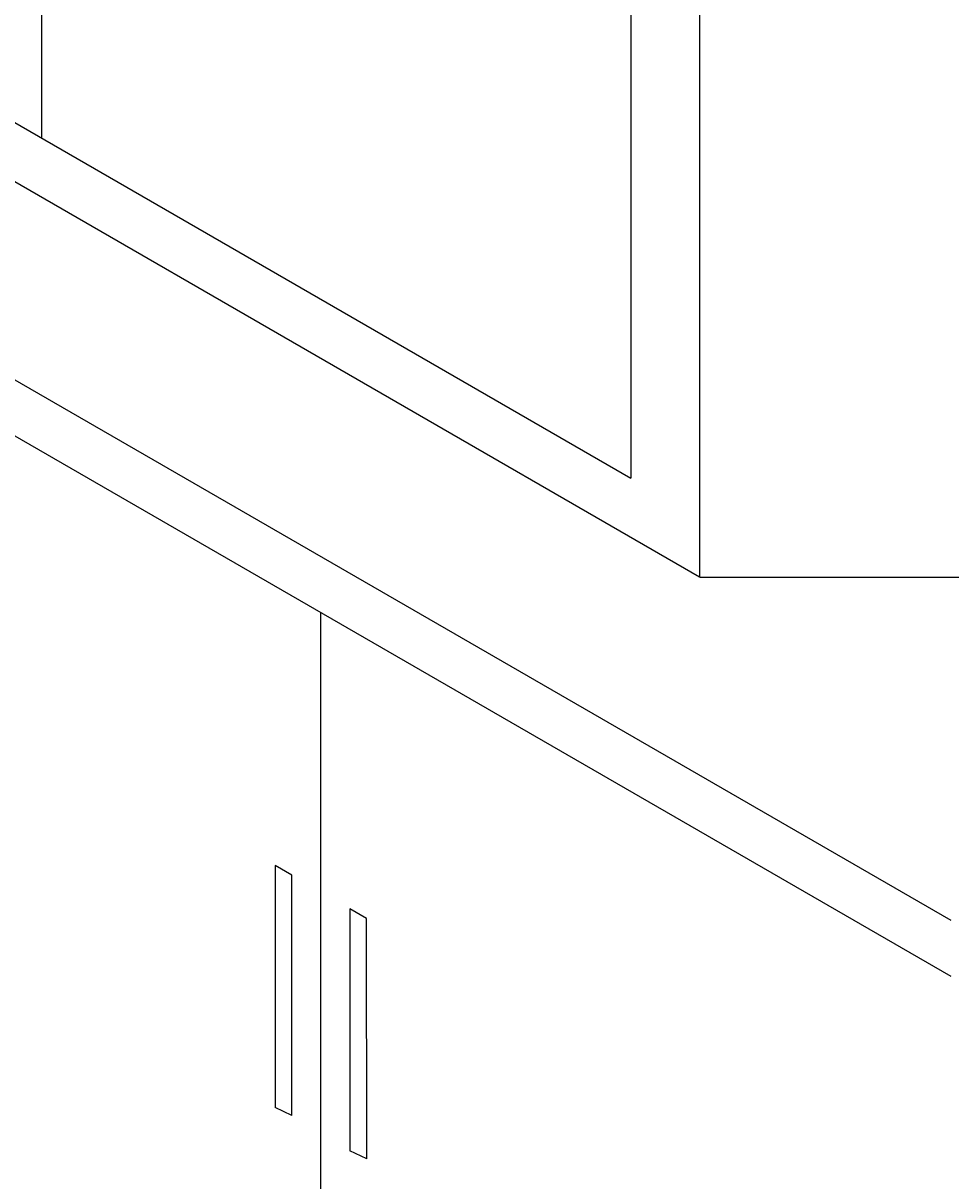
# Model space of a CAD drawing. Units: metres. Extents: x -2391 to 4922, y -635 to 4845.
# Tile 31 of 37: x 2198 to 3149, y 1238 to 2425. Entities that reach past the tile are written whole.
import ezdxf

# ---------------------------------------------------------------- set-up
doc = ezdxf.new("R2010")
doc.units = ezdxf.units.M
doc.header["$MEASUREMENT"] = 0
for name, color, linetype, lineweight in [('A-ANNO-DIMS', 2, 'Continuous', 18), ('A-FLOR-FIXT', 3, 'Continuous', 25), ('A-GLAZ', 4, 'Continuous', 25)]:
    doc.layers.add(name, color=color, linetype=linetype, lineweight=lineweight)
doc.styles.get("Standard").update_dxf_attribs({"font": 'arial.ttf'})
doc.dimstyles.get("Standard").update_dxf_attribs({"dimtxt": 5, "dimasz": 4, "dimexe": 0.18, "dimexo": 0.0625, "dimgap": 0.09, "dimtad": 0, "dimtih": 1, "dimtoh": 1, "dimdec": 0, "dimzin": 0, "dimdsep": 46, "dimtxsty": 'Standard', "dimcen": 0.09, "dimadec": 0, "dimazin": 0, "dimtfac": 1, "dimtdec": 0, "dimtofl": 0, "dimtmove": 0, "dimatfit": 3, "dimfxl": 1, "dimtolj": 1, "dimtzin": 0, "dimarcsym": 0})

# ---------------------------------------------------------------- blocks, each defined once
blk = doc.blocks.new('HANDLE-DOOR-256')
for p, q in [((0, 256.1), (0, 9.9)), ((0, 256.1), (17.1, 248)), ((17.1, 0), (17.1, 248)), ((0, 9.9), (17.1, 0))]:
    blk.add_line(p, q)
blk = doc.blocks.new('*D8')
at = {"layer": 'A-ANNO-DIMS', "color": 0, "lineweight": -2, "transparency": 16777216}
for p, q in [((-2047.3, 3005.2), (-2047.3, -631.4)), ((4577.8, 2350.2), (4577.8, -631.4)), ((-2043.3, -631.2), (1257.6, -631.2)), ((4573.8, -631.2), (1272.8, -631.2))]:
    blk.add_line(p, q, dxfattribs=at)
at = {"layer": 'A-ANNO-DIMS', "color": 0, "transparency": 16777216}
for points in [[(-2043.3, -630.6), (-2043.3, -631.9), (-2047.3, -631.2)], [(4573.8, -630.6), (4573.8, -631.9), (4577.8, -631.2)]]:
    blk.add_solid(points, dxfattribs=at)
at = {"layer": 'Defpoints', "color": 0, "transparency": 16777216}
for p in [(-2047.3, 3005.3), (4577.8, 2350.3), (4577.8, -631.2)]:
    blk.add_point(p, dxfattribs=at)
at = {"layer": 'A-ANNO-DIMS', "color": 0, "transparency": 16777216, "insert": (1265.2, -631.2), "char_height": 5, "attachment_point": 5}
blk.add_mtext('\\A1;6625', dxfattribs=at)
blk = doc.blocks.new('*D13')
at = {"layer": 'A-ANNO-DIMS', "color": 0, "lineweight": -2, "transparency": 16777216}
for p, q in [((2891.5, 2774), (3228.1, 2774)), ((3227.9, 2770), (3227.9, 2318)), ((3227.9, 1860.8), (3227.9, 2312.8)), ((2891.5, 1856.8), (3228.1, 1856.8))]:
    blk.add_line(p, q, dxfattribs=at)
at = {"layer": 'A-ANNO-DIMS', "color": 0, "transparency": 16777216}
for points in [[(3227.3, 2770), (3228.6, 2770), (3227.9, 2774)], [(3227.3, 1860.8), (3228.6, 1860.8), (3227.9, 1856.8)]]:
    blk.add_solid(points, dxfattribs=at)
at = {"layer": 'Defpoints', "color": 0, "transparency": 16777216}
for p in [(2891.4, 2774), (2891.4, 1856.8), (3227.9, 1856.8)]:
    blk.add_point(p, dxfattribs=at)
at = {"layer": 'A-ANNO-DIMS', "color": 0, "transparency": 16777216, "insert": (3227.9, 2315.4), "char_height": 5, "attachment_point": 5}
blk.add_mtext('\\A1;917.2', dxfattribs=at)

msp = doc.modelspace()

# ---------------------------------------------------------------- linework, layer by layer
at = {"layer": 'A-FLOR-FIXT'}
for p, q in [((550.7419, 3005.2763), (3148.8181, 1505.2763)), ((546.8938, 2950.1416), (3148.8181, 1447.9199)), ((2503.0469, 1820.756), (2503.0469, 998.1124))]:
    msp.add_line(p, q, dxfattribs=at)
at = {"layer": 'A-GLAZ'}
for p, q in [((2217.2021, 3091.6502), (2217.2021, 2306.7949)), ((2891.4324, 2773.9801), (2891.4324, 1856.8211)), ((2820.8768, 2743.1184), (2820.8768, 1958.2631)), ((1573.5273, 2678.4207), (2820.8768, 1958.2631)), ((2891.4324, 1856.8211), (1496.0309, 2662.4566))]:
    msp.add_line(p, q, dxfattribs=at)

# ---------------------------------------------------------------- block references
at = {"layer": 'A-FLOR-FIXT', "rotation": 180.0273381069543}
for p in [(2473.5093, 1561.1461), (2550.1961, 1516.8709)]:
    msp.add_blockref('HANDLE-DOOR-256', p, dxfattribs=at)

# ---------------------------------------------------------------- dimensions: what is measured, and where the dimension line sits
at = {"layer": 'A-ANNO-DIMS'}
dim = msp.add_linear_dim(base=(4577.76, -631.2237), p1=(-2047.3343, 3005.2763), p2=(4577.76, 2350.2763), dimstyle='Standard', override={"dimdec": 0, "dimlfac": 1, "dimrnd": 0, "dimzin": 0, "dimdsep": 46, "dimlunit": 2}, dxfattribs=at)
dim.commit()
dim.dimension.update_dxf_attribs({"geometry": '*D8', "text_midpoint": (1265.2128, -631.2237)})
dim = msp.add_linear_dim(base=(3227.9324, 1856.8211), p1=(2891.4324, 2773.9801), p2=(2891.4324, 1856.8211), angle=270, dimstyle='Standard', override={"dimdec": 1, "dimlfac": 1, "dimrnd": 0, "dimzin": 0, "dimdsep": 46, "dimlunit": 2}, dxfattribs=at)
dim.commit()
dim.dimension.update_dxf_attribs({"geometry": '*D13', "text_midpoint": (3227.9324, 2315.4006)})

doc.saveas('drawing.dxf')
